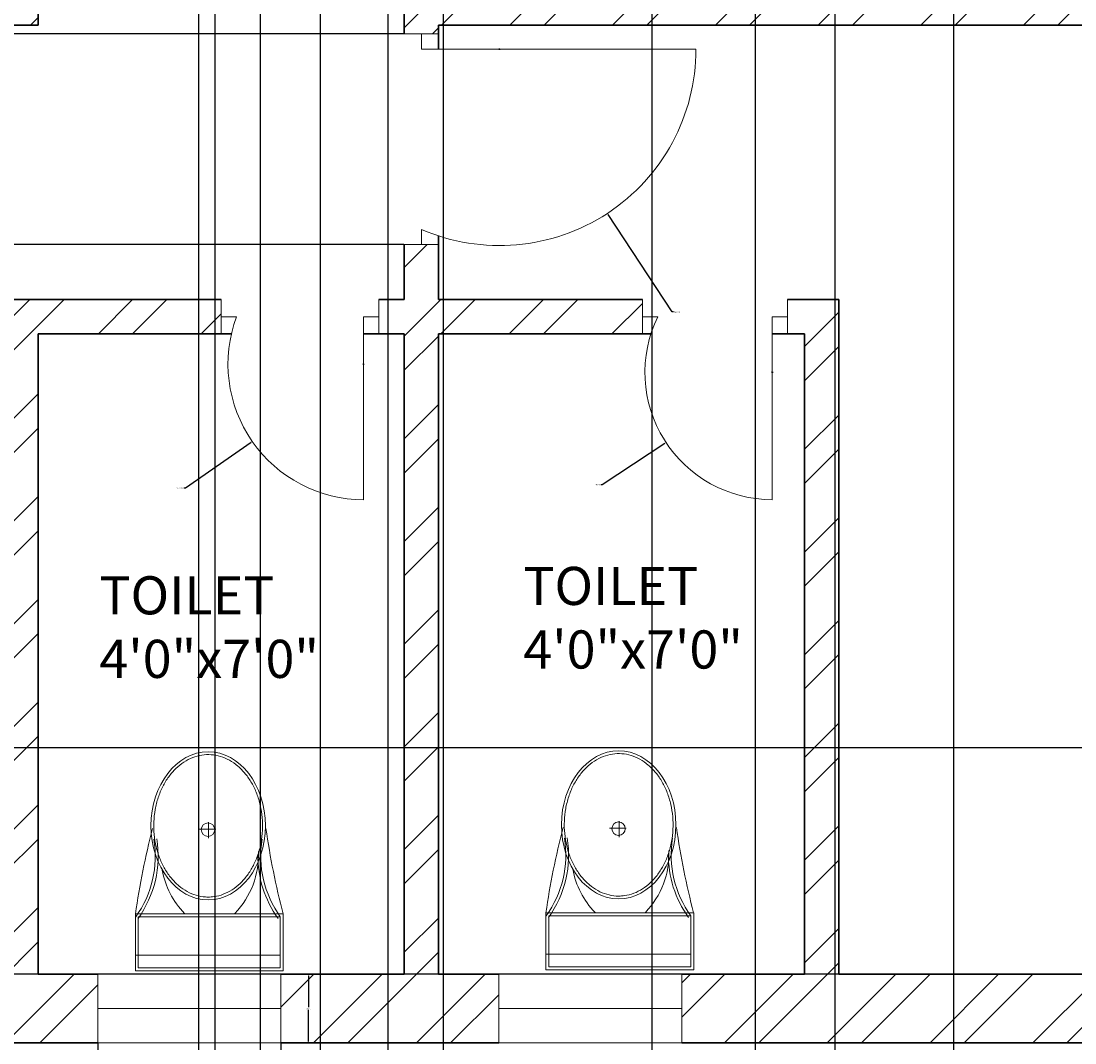
# Model space of a CAD drawing. Units: inches. Extents: x 1748 to 2382, y 1346 to 2284.
# Tile 4 of 26: x 2009 to 2147, y 1468 to 1602. Entities that reach past the tile are written whole.
import ezdxf

# ---------------------------------------------------------------- set-up
doc = ezdxf.new("R2010")
doc.units = ezdxf.units.IN
for name, color, linetype, lineweight in [('A-ANNO-DIMS', 2, 'Continuous', 18), ('A-AREA-IDEN', 7, 'Continuous', 18), ('A-DOOR', 21, 'Continuous', 18), ('A-FLOR-FIXT', 7, 'Continuous', 18), ('A-GLAZ', 191, 'Continuous', 18), ('A-WALL', 7, 'Continuous', 35), ('A-WALL-PATT', 9, 'Continuous', 13)]:
    doc.layers.add(name, color=color, linetype=linetype, lineweight=lineweight)
doc.styles.get("Standard").update_dxf_attribs({"font": 'arial.ttf'})
doc.dimstyles.get("Standard").update_dxf_attribs({"dimtxt": 0.18, "dimasz": 0.18, "dimexe": 0.18, "dimexo": 0.0625, "dimgap": 0.09, "dimtad": 0, "dimtih": 1, "dimtoh": 1, "dimdec": 4, "dimzin": 0, "dimdsep": 46, "dimtxsty": 'Standard', "dimcen": 0.09, "dimadec": 0, "dimazin": 0, "dimtfac": 1, "dimtdec": 4, "dimtofl": 0, "dimtmove": 0, "dimatfit": 3, "dimfxl": 1, "dimtolj": 1, "dimtzin": 0, "dimarcsym": 0})

# ---------------------------------------------------------------- blocks, each defined once
blk = doc.blocks.new('A$C31115884')
for p, q in [((257.5, 466.4), (257.5, 523.2)), ((283.1, 497.7), (223.4, 497.7)), ((0, 200), (0, 0)), ((520, 200), (0, 200)), ((10, 190), (10, 10)), ((510, 190), (10, 190)), ((510, 10), (510, 190)), ((520, 0), (520, 200)), ((510, 54.5), (0, 54.5)), ((10, 10), (510, 10)), ((0, 0), (520, 0))]:
    blk.add_line(p, q)
blk.add_circle((255.6, 496.4), 23.6)
for centre, radius, start, end in [((2777.7, -204.6), 2807, 165.4549, 171.7133), ((3237, 905), 2807, 188.2867, 194.5451), ((-294.5, 403.3), 364.7, 324.2091, 9.3499), ((-294.5, 403.3), 374.7, 324.2091, 9.3499), ((805.8, 403.3), 364.7, 170.6501, 215.7909), ((139.5, 406.2), 293.5, 315.8436, 2.6563), ((805.8, 403.3), 374.7, 179.2036, 215.7909), ((383.6, 406.2), 293.5, 190.2774, 224.1564)]:
    blk.add_arc(centre, radius, start, end)
blk.add_ellipse((256.2, 509.9), major_axis=(0, -260.7), ratio=0.772727)
blk.add_open_spline([(256.2, 259.2), (263.1, 259.2), (270, 259.7), (287.8, 262.3), (298.7, 265.1), (319.9, 273.1), (330.2, 278.4), (350.1, 291.1), (359.7, 298.7), (377.7, 315.9), (386.2, 325.5), (401.7, 346.6), (408.8, 358.1), (421.3, 382.5), (426.8, 395.5), (435.9, 422.4), (439.5, 436.4), (444.8, 465.1), (446.5, 479.7), (447.9, 509.2), (447.6, 524), (445, 553.3), (442.7, 567.8), (436.3, 596), (432.1, 609.7), (421.9, 636), (416, 648.6), (402.5, 672.1), (395, 683), (378.6, 703), (369.8, 712.1), (351.1, 728), (341.3, 734.8), (320.9, 746.2), (310.4, 750.7), (288.9, 757.3), (278, 759.4), (256, 761), (245, 760.6), (223.1, 757.2), (212.3, 754.3), (191.1, 746.1), (180.8, 740.7), (160.9, 727.8), (151.4, 720.1), (133.5, 702.7), (125.1, 693), (109.6, 671.7), (102.6, 660.2), (90.2, 635.7), (84.9, 622.7), (76, 595.6), (72.4, 581.6), (67.2, 552.9), (65.6, 538.2), (64.4, 508.8), (64.8, 494), (67.5, 464.7), (69.9, 450.2), (76.6, 422), (80.8, 408.3), (91.1, 382.2), (97.2, 369.7), (110.8, 346.3), (118.4, 335.4), (134.8, 315.6), (143.7, 306.7), (162.4, 290.9), (172.3, 284.2), (192.8, 273), (203.3, 268.6), (224.8, 262.2), (235.8, 260.2), (249.9, 259.3), (253, 259.2), (256.2, 259.2)], degree=3, knots=[0, 0, 0, 0, 0.110105, 0.110105, 0.285049, 0.285049, 0.459994, 0.459994, 0.634938, 0.634938, 0.809882, 0.809882, 0.984827, 0.984827, 1.159771, 1.159771, 1.334715, 1.334715, 1.50966, 1.50966, 1.684604, 1.684604, 1.859549, 1.859549, 2.034493, 2.034493, 2.209437, 2.209437, 2.384382, 2.384382, 2.559326, 2.559326, 2.73427, 2.73427, 2.909215, 2.909215, 3.084159, 3.084159, 3.259103, 3.259103, 3.434048, 3.434048, 3.608992, 3.608992, 3.783936, 3.783936, 3.958881, 3.958881, 4.133825, 4.133825, 4.30877, 4.30877, 4.483714, 4.483714, 4.658658, 4.658658, 4.833603, 4.833603, 5.008547, 5.008547, 5.183491, 5.183491, 5.358436, 5.358436, 5.53338, 5.53338, 5.708324, 5.708324, 5.883269, 5.883269, 6.058213, 6.058213, 6.233158, 6.233158, 6.283185, 6.283185, 6.283185, 6.283185])
blk = doc.blocks.new('WIN-24-DEEP')
for p, q in [((0, 9), (0, 0)), ((0, 9), (24, 9)), ((24, 4.5), (24, 9)), ((24, 9), (24, 0)), ((0, 0), (0, 4.5)), ((0, 4.5), (24, 4.5)), ((24, 0), (0, 0))]:
    blk.add_line(p, q)
blk = doc.blocks.new('*D32')
at = {"layer": 'A-ANNO-DIMS', "color": 0, "lineweight": -2, "transparency": 16777216}
for p, q in [((2018.79, 1467.79), (2018.79, 1464.07)), ((2042.79, 1467.79), (2042.79, 1464.07)), ((2018.97, 1464.25), (2029.67, 1464.25)), ((2042.61, 1464.25), (2031.91, 1464.25))]:
    blk.add_line(p, q, dxfattribs=at)
at = {"layer": 'A-ANNO-DIMS', "color": 0, "transparency": 16777216}
for points in [[(2018.97, 1464.28), (2018.97, 1464.22), (2018.79, 1464.25)], [(2042.61, 1464.28), (2042.61, 1464.22), (2042.79, 1464.25)]]:
    blk.add_solid(points, dxfattribs=at)
at = {"layer": 'Defpoints', "color": 0, "transparency": 16777216}
for p in [(2018.79, 1467.85), (2042.79, 1467.85), (2042.79, 1464.25)]:
    blk.add_point(p, dxfattribs=at)
at = {"layer": 'A-ANNO-DIMS', "color": 0, "transparency": 16777216, "insert": (2030.79, 1464.25), "char_height": 0.18, "attachment_point": 5}
blk.add_mtext('\\A1;WINDOW 24 TYP.', dxfattribs=at)
blk = doc.blocks.new('*D33')
at = {"layer": 'A-ANNO-DIMS', "color": 0, "lineweight": -2, "transparency": 16777216}
for p, q in [((2042.85, 1476.85), (2046.57, 1476.85)), ((2046.39, 1476.67), (2046.39, 1472.53)), ((2046.39, 1468.03), (2046.39, 1472.17)), ((2042.85, 1467.85), (2046.57, 1467.85))]:
    blk.add_line(p, q, dxfattribs=at)
at = {"layer": 'A-ANNO-DIMS', "color": 0, "transparency": 16777216}
for points in [[(2046.36, 1476.67), (2046.42, 1476.67), (2046.39, 1476.85)], [(2046.36, 1468.03), (2046.42, 1468.03), (2046.39, 1467.85)]]:
    blk.add_solid(points, dxfattribs=at)
at = {"layer": 'Defpoints', "color": 0, "transparency": 16777216}
for p in [(2042.79, 1476.85), (2046.39, 1476.85), (2042.79, 1467.85)]:
    blk.add_point(p, dxfattribs=at)
at = {"layer": 'A-ANNO-DIMS', "color": 0, "transparency": 16777216, "insert": (2046.39, 1472.35), "char_height": 0.18, "attachment_point": 5}
blk.add_mtext('\\A1;9 TYP.', dxfattribs=at)
blk = doc.blocks.new('*D36')
at = {"layer": 'A-ANNO-DIMS', "color": 0, "lineweight": -2, "transparency": 16777216}
for p, q in [((2031.96, 1970.29), (2031.96, 1360.47)), ((2130.96, 1970.29), (2130.96, 1360.47)), ((2032.14, 1360.65), (2081.24, 1360.65)), ((2130.78, 1360.65), (2081.68, 1360.65))]:
    blk.add_line(p, q, dxfattribs=at)
at = {"layer": 'A-ANNO-DIMS', "color": 0, "transparency": 16777216}
for points in [[(2032.14, 1360.68), (2032.14, 1360.62), (2031.96, 1360.65)], [(2130.78, 1360.68), (2130.78, 1360.62), (2130.96, 1360.65)]]:
    blk.add_solid(points, dxfattribs=at)
at = {"layer": 'Defpoints', "color": 0, "transparency": 16777216}
for p in [(2031.96, 1970.35), (2130.96, 1970.35), (2130.96, 1360.65)]:
    blk.add_point(p, dxfattribs=at)
at = {"layer": 'A-ANNO-DIMS', "color": 0, "transparency": 16777216, "insert": (2081.46, 1360.65), "char_height": 0.18, "attachment_point": 5}
blk.add_mtext('\\A1;99', dxfattribs=at)
blk = doc.blocks.new('*D51')
at = {"layer": 'A-ANNO-DIMS', "color": 0, "lineweight": -2, "transparency": 16777216}
for p, q in [((1968.44, 2223.79), (1968.44, 1360.47)), ((2040.07, 2223.79), (2040.07, 1360.47)), ((1968.62, 1360.65), (2003.86, 1360.65)), ((2039.89, 1360.65), (2004.65, 1360.65))]:
    blk.add_line(p, q, dxfattribs=at)
at = {"layer": 'A-ANNO-DIMS', "color": 0, "transparency": 16777216}
for points in [[(1968.62, 1360.68), (1968.62, 1360.62), (1968.44, 1360.65)], [(2039.89, 1360.68), (2039.89, 1360.62), (2040.07, 1360.65)]]:
    blk.add_solid(points, dxfattribs=at)
at = {"layer": 'Defpoints', "color": 0, "transparency": 16777216}
for p in [(1968.44, 2223.85), (2040.07, 2223.85), (2040.07, 1360.65)]:
    blk.add_point(p, dxfattribs=at)
at = {"layer": 'A-ANNO-DIMS', "color": 0, "transparency": 16777216, "insert": (2004.26, 1360.65), "char_height": 0.18, "attachment_point": 5}
blk.add_mtext('\\A1;71.62', dxfattribs=at)
blk = doc.blocks.new('*D52')
at = {"layer": 'A-ANNO-DIMS', "color": 0, "lineweight": -2, "transparency": 16777216}
for p, q in [((2064.07, 2223.79), (2064.07, 1360.47)), ((2091.4, 2223.79), (2091.4, 1360.47)), ((2064.25, 1360.65), (2077.34, 1360.65)), ((2091.22, 1360.65), (2078.13, 1360.65))]:
    blk.add_line(p, q, dxfattribs=at)
at = {"layer": 'A-ANNO-DIMS', "color": 0, "transparency": 16777216}
for points in [[(2064.25, 1360.68), (2064.25, 1360.62), (2064.07, 1360.65)], [(2091.22, 1360.68), (2091.22, 1360.62), (2091.4, 1360.65)]]:
    blk.add_solid(points, dxfattribs=at)
at = {"layer": 'Defpoints', "color": 0, "transparency": 16777216}
for p in [(2064.07, 2223.85), (2091.4, 2223.85), (2091.4, 1360.65)]:
    blk.add_point(p, dxfattribs=at)
at = {"layer": 'A-ANNO-DIMS', "color": 0, "transparency": 16777216, "insert": (2077.73, 1360.65), "char_height": 0.18, "attachment_point": 5}
blk.add_mtext('\\A1;27.33', dxfattribs=at)
blk = doc.blocks.new('*D53')
at = {"layer": 'A-ANNO-DIMS', "color": 0, "lineweight": -2, "transparency": 16777216}
for p, q in [((2115.4, 2223.79), (2115.4, 1360.47)), ((2167.02, 2223.79), (2167.02, 1360.47)), ((2115.58, 1360.65), (2140.81, 1360.65)), ((2166.84, 1360.65), (2141.6, 1360.65))]:
    blk.add_line(p, q, dxfattribs=at)
at = {"layer": 'A-ANNO-DIMS', "color": 0, "transparency": 16777216}
for points in [[(2115.58, 1360.68), (2115.58, 1360.62), (2115.4, 1360.65)], [(2166.84, 1360.68), (2166.84, 1360.62), (2167.02, 1360.65)]]:
    blk.add_solid(points, dxfattribs=at)
at = {"layer": 'Defpoints', "color": 0, "transparency": 16777216}
for p in [(2115.4, 2223.85), (2167.02, 2223.85), (2167.02, 1360.65)]:
    blk.add_point(p, dxfattribs=at)
at = {"layer": 'A-ANNO-DIMS', "color": 0, "transparency": 16777216, "insert": (2141.21, 1360.65), "char_height": 0.18, "attachment_point": 5}
blk.add_mtext('\\A1;51.62', dxfattribs=at)
blk = doc.blocks.new('*D54')
at = {"layer": 'A-ANNO-DIMS', "color": 0, "lineweight": -2, "transparency": 16777216}
for p, q in [((2288.4, 1506.57), (1779.88, 1506.57)), ((1780.06, 1506.39), (1780.06, 1491.89)), ((1780.06, 1477.03), (1780.06, 1491.53)), ((2288.4, 1476.85), (1779.88, 1476.85))]:
    blk.add_line(p, q, dxfattribs=at)
at = {"layer": 'A-ANNO-DIMS', "color": 0, "transparency": 16777216}
for points in [[(1780.03, 1506.39), (1780.09, 1506.39), (1780.06, 1506.57)], [(1780.03, 1477.03), (1780.09, 1477.03), (1780.06, 1476.85)]]:
    blk.add_solid(points, dxfattribs=at)
at = {"layer": 'Defpoints', "color": 0, "transparency": 16777216}
for p in [(1780.06, 1506.57), (2288.46, 1506.57), (2288.46, 1476.85)]:
    blk.add_point(p, dxfattribs=at)
at = {"layer": 'A-ANNO-DIMS', "color": 0, "transparency": 16777216, "insert": (1780.06, 1491.71), "char_height": 0.18, "attachment_point": 5}
blk.add_mtext('\\A1;29.716', dxfattribs=at)
blk = doc.blocks.new('*D61')
at = {"layer": 'A-ANNO-DIMS', "color": 0, "lineweight": -2, "transparency": 16777216}
for p, q in [((2047.92, 1854.79), (2047.92, 1360.47)), ((2104.96, 1854.79), (2104.96, 1360.47)), ((2048.1, 1360.65), (2076.04, 1360.65)), ((2104.78, 1360.65), (2076.83, 1360.65))]:
    blk.add_line(p, q, dxfattribs=at)
at = {"layer": 'A-ANNO-DIMS', "color": 0, "transparency": 16777216}
for points in [[(2048.1, 1360.68), (2048.1, 1360.62), (2047.92, 1360.65)], [(2104.78, 1360.68), (2104.78, 1360.62), (2104.96, 1360.65)]]:
    blk.add_solid(points, dxfattribs=at)
at = {"layer": 'Defpoints', "color": 0, "transparency": 16777216}
for p in [(2047.92, 1854.85), (2104.96, 1854.85), (2104.96, 1360.65)]:
    blk.add_point(p, dxfattribs=at)
at = {"layer": 'A-ANNO-DIMS', "color": 0, "transparency": 16777216, "insert": (2076.44, 1360.65), "char_height": 0.18, "attachment_point": 5}
blk.add_mtext('\\A1;57.04', dxfattribs=at)
blk = doc.blocks.new('*D78')
at = {"layer": 'A-ANNO-DIMS', "color": 0, "lineweight": -2, "transparency": 16777216}
for p, q in [((2034.13, 2132.54), (2034.13, 1360.47)), ((2056.8, 2127.06), (2056.8, 1360.47)), ((2034.31, 1360.65), (2045, 1360.65)), ((2056.62, 1360.65), (2045.93, 1360.65))]:
    blk.add_line(p, q, dxfattribs=at)
at = {"layer": 'A-ANNO-DIMS', "color": 0, "transparency": 16777216}
for points in [[(2034.31, 1360.68), (2034.31, 1360.62), (2034.13, 1360.65)], [(2056.62, 1360.68), (2056.62, 1360.62), (2056.8, 1360.65)]]:
    blk.add_solid(points, dxfattribs=at)
at = {"layer": 'Defpoints', "color": 0, "transparency": 16777216}
for p in [(2034.13, 2132.6), (2056.8, 2127.13), (2056.8, 1360.65)]:
    blk.add_point(p, dxfattribs=at)
at = {"layer": 'A-ANNO-DIMS', "color": 0, "transparency": 16777216, "insert": (2045.47, 1360.65), "char_height": 0.18, "attachment_point": 5}
blk.add_mtext('\\A1;22.663', dxfattribs=at)
blk = doc.blocks.new('*D80')
at = {"layer": 'A-ANNO-DIMS', "color": 0, "lineweight": -2, "transparency": 16777216}
for p, q in [((2058.9, 1600.19), (1779.88, 1600.19)), ((1780.06, 1600.01), (1780.06, 1586.55)), ((1780.06, 1572.73), (1780.06, 1586.19)), ((2058.9, 1572.55), (1779.88, 1572.55))]:
    blk.add_line(p, q, dxfattribs=at)
at = {"layer": 'A-ANNO-DIMS', "color": 0, "transparency": 16777216}
for points in [[(1780.03, 1600.01), (1780.09, 1600.01), (1780.06, 1600.19)], [(1780.03, 1572.73), (1780.09, 1572.73), (1780.06, 1572.55)]]:
    blk.add_solid(points, dxfattribs=at)
at = {"layer": 'Defpoints', "color": 0, "transparency": 16777216}
for p in [(1780.06, 1600.19), (2058.96, 1600.19), (2058.96, 1572.55)]:
    blk.add_point(p, dxfattribs=at)
at = {"layer": 'A-ANNO-DIMS', "color": 0, "transparency": 16777216, "insert": (1780.06, 1586.37), "char_height": 0.18, "attachment_point": 5}
blk.add_mtext('\\A1;27.637', dxfattribs=at)
blk = doc.blocks.new('*D86')
at = {"layer": 'A-ANNO-DIMS', "color": 0, "lineweight": -2, "transparency": 16777216}
for p, q in [((2071.36, 1598.19), (2071.54, 1598.19)), ((2071.45, 1598.1), (2071.45, 1598.28)), ((2094.07, 1563.73), (2085.69, 1576.5)), ((2094.25, 1563.73), (2094.07, 1563.73))]:
    blk.add_line(p, q, dxfattribs=at)
at = {"layer": 'A-ANNO-DIMS', "color": 0, "transparency": 16777216}
blk.add_solid([(2085.71, 1576.52), (2085.66, 1576.49), (2085.59, 1576.65)], dxfattribs=at)
at = {"layer": 'Defpoints', "color": 0, "transparency": 16777216}
for p in [(2071.45, 1598.19), (2085.59, 1576.65)]:
    blk.add_point(p, dxfattribs=at)
at = {"layer": 'A-ANNO-DIMS', "color": 0, "transparency": 16777216, "insert": (2094.73, 1563.73), "char_height": 0.18, "attachment_point": 5}
blk.add_mtext('\\A1;R25.76', dxfattribs=at)
blk = doc.blocks.new('*D92')
at = {"layer": 'A-ANNO-DIMS', "color": 0, "lineweight": -2, "transparency": 16777216}
for p, q in [((2053.54, 1556.89), (2053.72, 1556.89)), ((2053.63, 1556.8), (2053.63, 1556.98)), ((2030.25, 1540.65), (2038.87, 1546.64)), ((2030.07, 1540.65), (2030.25, 1540.65))]:
    blk.add_line(p, q, dxfattribs=at)
at = {"layer": 'A-ANNO-DIMS', "color": 0, "transparency": 16777216}
blk.add_solid([(2038.85, 1546.66), (2038.89, 1546.61), (2039.02, 1546.74)], dxfattribs=at)
at = {"layer": 'Defpoints', "color": 0, "transparency": 16777216}
for p in [(2053.63, 1556.89), (2039.02, 1546.74)]:
    blk.add_point(p, dxfattribs=at)
at = {"layer": 'A-ANNO-DIMS', "color": 0, "transparency": 16777216, "insert": (2029.52, 1540.65), "char_height": 0.18, "attachment_point": 5}
blk.add_mtext('\\A1;R17.788', dxfattribs=at)
blk = doc.blocks.new('*D96')
at = {"layer": 'A-ANNO-DIMS', "color": 0, "lineweight": -2, "transparency": 16777216}
for p, q in [((2107.13, 1555.81), (2107.31, 1555.81)), ((2107.22, 1555.72), (2107.22, 1555.9)), ((2084.92, 1541.07), (2093.13, 1546.5)), ((2084.74, 1541.07), (2084.92, 1541.07))]:
    blk.add_line(p, q, dxfattribs=at)
at = {"layer": 'A-ANNO-DIMS', "color": 0, "transparency": 16777216}
blk.add_solid([(2093.11, 1546.52), (2093.15, 1546.47), (2093.28, 1546.59)], dxfattribs=at)
at = {"layer": 'Defpoints', "color": 0, "transparency": 16777216}
for p in [(2107.22, 1555.81), (2093.28, 1546.59)]:
    blk.add_point(p, dxfattribs=at)
at = {"layer": 'A-ANNO-DIMS', "color": 0, "transparency": 16777216, "insert": (2084.28, 1541.07), "char_height": 0.18, "attachment_point": 5}
blk.add_mtext('\\A1;R16.71', dxfattribs=at)

msp = doc.modelspace()

# ---------------------------------------------------------------- hatches: boundary and pattern name
at = {"layer": 'A-WALL-PATT'}
h = msp.add_hatch(dxfattribs=at)
h.set_pattern_fill('ANSI32', color=256)
h.paths.add_polyline_path([(1908.4445, 2232.8497), (1821.9607, 2232.8497), (1821.9607, 2223.8497), (1865.4607, 2223.8497), (1865.4607, 2209.9185), (1869.9607, 2209.9185), (1869.9607, 2223.8497), (1908.4445, 2223.8497), (1908.4445, 2228.3497)])
h.paths.add_polyline_path([(2040.0683, 2232.8497), (1968.4445, 2232.8497), (1968.4445, 2223.8497), (2025.9607, 2223.8497), (2025.9607, 2130.3497), (2032.1341, 2130.3497), (2032.1341, 2132.5997), (2032.1341, 2134.8497), (2030.4607, 2134.8497), (2030.4607, 2223.8497), (2040.0683, 2223.8497)])
h.paths.add_polyline_path([(2091.3969, 2232.8497), (2064.0683, 2232.8497), (2064.0683, 2223.8497), (2078.4607, 2223.8497), (2078.4607, 2134.8497), (2051.1563, 2134.8497), (2051.1563, 2130.3497), (2078.4607, 2130.3497), (2078.4607, 2128.6813), (2082.9607, 2128.6813), (2082.9607, 2130.3497), (2086.1879, 2130.3497), (2086.1879, 2132.5997), (2086.1879, 2134.8497), (2082.9607, 2134.8497), (2082.9607, 2223.8497), (2091.3969, 2223.8497), (2091.3969, 2228.3497)])
h.paths.add_polyline_path([(2167.0164, 2232.8497), (2115.3969, 2232.8497), (2115.3969, 2223.8497), (2130.9607, 2223.8497), (2130.9607, 2134.8497), (2106.9607, 2134.8497), (2106.9607, 2130.3497), (2135.4607, 2130.3497), (2135.4607, 2223.8497), (2167.0164, 2223.8497), (2167.0164, 2228.3497)])
h.paths.add_polyline_path([(1869.9607, 2149.9185), (1865.4607, 2149.9185), (1865.4607, 2127.8942), (1869.9607, 2127.8942)])
h.paths.add_polyline_path([(2082.9607, 2104.4871), (2080.7107, 2104.4871), (2078.4607, 2104.4871), (2078.4607, 2103.8497), (1869.9607, 2103.8497), (1869.9607, 2108.6062), (1867.7107, 2108.6062), (1865.4607, 2108.6062), (1865.4607, 2103.8497), (1821.9607, 2103.8497), (1821.9607, 2099.3497), (1865.4607, 2099.3497), (1865.4607, 2094.7509), (1869.9607, 2094.7509), (1869.9607, 2099.3497), (2025.9607, 2099.3497), (2025.9607, 2096.4326), (2030.4607, 2096.4326), (2030.4607, 2099.3497), (2082.9607, 2099.3497)])
h.paths.add_polyline_path([(1928.9457, 1401.1212), (2176.8693, 1401.1212), (2176.8693, 1438.214), (1928.9457, 1438.214)], flags=9)
h.paths.add_polyline_path([(2122.2668, 2048.1927), (2177.9387, 2048.1927), (2177.9387, 2066.85), (2122.2668, 2066.85)], flags=9)
h.paths.add_polyline_path([(2272.688, 2153.8197), (2272.688, 2216.746), (2262.3845, 2216.746), (2262.3845, 2153.8197)], flags=9)
h.paths.add_polyline_path([(2157.2928, 2166.5593), (2196.3822, 2166.5593), (2196.3822, 2185.2167), (2157.2928, 2185.2167)], flags=9)
h.paths.add_polyline_path([(2089.3407, 2162.0698), (2124.3987, 2162.0698), (2124.3987, 2180.7272), (2089.3407, 2180.7272)], flags=9)
h.paths.add_polyline_path([(2037.4521, 2160.0913), (2072.5101, 2160.0913), (2072.5101, 2178.7486), (2037.4521, 2178.7486)], flags=9)
h.paths.add_polyline_path([(1884.7894, 2104.1554), (1923.6297, 2104.1554), (1923.6297, 2122.8127), (1884.7894, 2122.8127)], flags=9)
h.paths.add_polyline_path([(1851.2832, 2142.9749), (1851.2832, 2199.3051), (1840.9796, 2199.3051), (1840.9796, 2142.9749)], flags=9)
h.paths.add_polyline_path([(1844.8763, 2017.2834), (1844.8763, 2073.6136), (1834.5728, 2073.6136), (1834.5728, 2017.2834)], flags=9)
h.paths.add_polyline_path([(1897.1577, 2073.1279), (1935.9981, 2073.1279), (1935.9981, 2091.7853), (1897.1577, 2091.7853)], flags=9)
h.paths.add_polyline_path([(1952.3395, 1802.4231), (2008.0114, 1802.4231), (2008.0114, 1821.0805), (1952.3395, 1821.0805)], flags=9)
h.paths.add_polyline_path([(1978.8184, 1857.6841), (2017.7338, 1857.6841), (2017.7338, 1876.3415), (1978.8184, 1876.3415)], flags=9)
h.paths.add_polyline_path([(1979.6513, 1925.9516), (2008.8089, 1925.9516), (2008.8089, 1944.6089), (1979.6513, 1944.6089)], flags=9)
h.paths.add_polyline_path([(1838.5553, 1860.3527), (1877.3957, 1860.3527), (1877.3957, 1879.01), (1838.5553, 1879.01)], flags=9)
h.paths.add_polyline_path([(1883.9018, 1787.3013), (1883.9018, 1843.6315), (1873.5983, 1843.6315), (1873.5983, 1787.3013)], flags=9)
h.paths.add_polyline_path([(1873.7079, 1509.1938), (1873.7079, 1583.7709), (1863.4044, 1583.7709), (1863.4044, 1509.1938)], flags=9)
h.paths.add_polyline_path([(1916.2259, 1603.3681), (1955.0663, 1603.3681), (1955.0663, 1622.0254), (1916.2259, 1622.0254)], flags=9)
h.paths.add_polyline_path([(1876.3013, 1636.757), (1876.3013, 1693.0871), (1865.9978, 1693.0871), (1865.9978, 1636.757)], flags=9)
h.paths.add_polyline_path([(1921.3138, 1521.8316), (1964.0662, 1521.8316), (1964.0662, 1540.489), (1921.3138, 1540.489)], flags=9)
h.paths.add_polyline_path([(2017.5657, 1497.5078), (2046.7983, 1497.5078), (2046.7983, 1516.1651), (2017.5657, 1516.1651)], flags=9)
h.paths.add_polyline_path([(2066.8661, 1499.3902), (2096.0988, 1499.3902), (2096.0988, 1518.0475), (2066.8661, 1518.0475)], flags=9)
h.paths.add_polyline_path([(2155.4835, 1571.6596), (2198.2358, 1571.6596), (2198.2358, 1590.3169), (2155.4835, 1590.3169)], flags=9)
h.paths.add_polyline_path([(2094.9136, 1664.6812), (2150.5855, 1664.6812), (2150.5855, 1683.3386), (2094.9136, 1683.3386)], flags=9)
h.paths.add_polyline_path([(2257.6902, 1863.1628), (2269.8935, 1863.1628), (2269.8935, 1873.4664), (2257.6902, 1873.4664)], flags=9)
h.paths.add_polyline_path([(2164.0748, 1880.3089), (2189.8694, 1880.3089), (2189.8694, 1890.6124), (2164.0748, 1890.6124)], flags=9)
h.paths.add_polyline_path([(2239.4394, 1931.0585), (2268.8187, 1931.0585), (2268.8187, 1949.7159), (2239.4394, 1949.7159)], flags=9)
h = msp.add_hatch(dxfattribs=at)
h.set_pattern_fill('ANSI32', color=256)
h.paths.add_polyline_path([(2297.4607, 2232.8497), (2203.0164, 2232.8497), (2203.0164, 2223.8497), (2244.9607, 2223.8497), (2244.9607, 2127.8554), (2249.4607, 2127.8554), (2249.4607, 2223.8497), (2297.4607, 2223.8497)])
h.paths.add_polyline_path([(2297.4607, 2103.8497), (2249.4607, 2103.8497), (2249.4607, 2106.7497), (2247.2107, 2106.7497), (2244.9607, 2106.7497), (2244.9607, 2103.8497), (2130.9607, 2103.8497), (2130.9607, 2099.3497), (2288.4607, 2099.3497), (2288.4607, 2077.2008), (2297.4607, 2077.2008)])
h.paths.add_polyline_path([(1928.9457, 1401.1212), (2176.8693, 1401.1212), (2176.8693, 1438.214), (1928.9457, 1438.214)], flags=9)
h.paths.add_polyline_path([(2122.2668, 2048.1927), (2177.9387, 2048.1927), (2177.9387, 2066.85), (2122.2668, 2066.85)], flags=9)
h.paths.add_polyline_path([(2272.688, 2153.8197), (2272.688, 2216.746), (2262.3845, 2216.746), (2262.3845, 2153.8197)], flags=25)
h.paths.add_polyline_path([(2157.2928, 2166.5593), (2196.3822, 2166.5593), (2196.3822, 2185.2167), (2157.2928, 2185.2167)], flags=9)
h.paths.add_polyline_path([(2089.3407, 2162.0698), (2124.3987, 2162.0698), (2124.3987, 2180.7272), (2089.3407, 2180.7272)], flags=9)
h.paths.add_polyline_path([(2037.4521, 2160.0913), (2072.5101, 2160.0913), (2072.5101, 2178.7486), (2037.4521, 2178.7486)], flags=9)
h.paths.add_polyline_path([(1884.7894, 2104.1554), (1923.6297, 2104.1554), (1923.6297, 2122.8127), (1884.7894, 2122.8127)], flags=9)
h.paths.add_polyline_path([(1851.2832, 2142.9749), (1851.2832, 2199.3051), (1840.9796, 2199.3051), (1840.9796, 2142.9749)], flags=9)
h.paths.add_polyline_path([(1844.8763, 2017.2834), (1844.8763, 2073.6136), (1834.5728, 2073.6136), (1834.5728, 2017.2834)], flags=9)
h.paths.add_polyline_path([(1897.1577, 2073.1279), (1935.9981, 2073.1279), (1935.9981, 2091.7853), (1897.1577, 2091.7853)], flags=9)
h.paths.add_polyline_path([(1952.3395, 1802.4231), (2008.0114, 1802.4231), (2008.0114, 1821.0805), (1952.3395, 1821.0805)], flags=9)
h.paths.add_polyline_path([(1978.8184, 1857.6841), (2017.7338, 1857.6841), (2017.7338, 1876.3415), (1978.8184, 1876.3415)], flags=9)
h.paths.add_polyline_path([(1979.6513, 1925.9516), (2008.8089, 1925.9516), (2008.8089, 1944.6089), (1979.6513, 1944.6089)], flags=9)
h.paths.add_polyline_path([(1838.5553, 1860.3527), (1877.3957, 1860.3527), (1877.3957, 1879.01), (1838.5553, 1879.01)], flags=9)
h.paths.add_polyline_path([(1883.9018, 1787.3013), (1883.9018, 1843.6315), (1873.5983, 1843.6315), (1873.5983, 1787.3013)], flags=9)
h.paths.add_polyline_path([(1873.7079, 1509.1938), (1873.7079, 1583.7709), (1863.4044, 1583.7709), (1863.4044, 1509.1938)], flags=9)
h.paths.add_polyline_path([(1916.2259, 1603.3681), (1955.0663, 1603.3681), (1955.0663, 1622.0254), (1916.2259, 1622.0254)], flags=9)
h.paths.add_polyline_path([(1876.3013, 1636.757), (1876.3013, 1693.0871), (1865.9978, 1693.0871), (1865.9978, 1636.757)], flags=9)
h.paths.add_polyline_path([(1921.3138, 1521.8316), (1964.0662, 1521.8316), (1964.0662, 1540.489), (1921.3138, 1540.489)], flags=9)
h.paths.add_polyline_path([(2017.5657, 1497.5078), (2046.7983, 1497.5078), (2046.7983, 1516.1651), (2017.5657, 1516.1651)], flags=9)
h.paths.add_polyline_path([(2066.8661, 1499.3902), (2096.0988, 1499.3902), (2096.0988, 1518.0475), (2066.8661, 1518.0475)], flags=9)
h.paths.add_polyline_path([(2155.4835, 1571.6596), (2198.2358, 1571.6596), (2198.2358, 1590.3169), (2155.4835, 1590.3169)], flags=9)
h.paths.add_polyline_path([(2094.9136, 1664.6812), (2150.5855, 1664.6812), (2150.5855, 1683.3386), (2094.9136, 1683.3386)], flags=9)
h.paths.add_polyline_path([(2257.6902, 1863.1628), (2269.8935, 1863.1628), (2269.8935, 1873.4664), (2257.6902, 1873.4664)], flags=9)
h.paths.add_polyline_path([(2164.0748, 1880.3089), (2189.8694, 1880.3089), (2189.8694, 1890.6124), (2164.0748, 1890.6124)], flags=9)
h.paths.add_polyline_path([(2239.4394, 1931.0585), (2268.8187, 1931.0585), (2268.8187, 1949.7159), (2239.4394, 1949.7159)], flags=9)
h = msp.add_hatch(dxfattribs=at)
h.set_pattern_fill('ANSI32', color=256)
h.paths.add_polyline_path([(1919.6777, 1476.8497), (1900.6426, 1476.8497), (1900.6426, 1522.0826), (1898.3926, 1522.0826), (1896.1426, 1522.0826), (1896.1426, 1476.8497), (1857.1426, 1476.8497), (1857.1426, 1467.8497), (1896.1426, 1467.8497), (1919.6777, 1467.8497), (1919.6777, 1472.3497)])
h.paths.add_polyline_path([(2018.7873, 1472.3497), (2018.7873, 1476.8497), (2010.9607, 1476.8497), (2010.9607, 1560.8497), (2034.9607, 1560.8497), (2034.9607, 1565.3497), (2006.4607, 1565.3497), (2006.4607, 1476.8497), (1955.6777, 1476.8497), (1955.6777, 1467.8497), (2018.7873, 1467.8497)])
h.paths.add_polyline_path([(2152.3354, 1472.3497), (2152.3354, 1476.8497), (2115.9607, 1476.8497), (2115.9607, 1565.3497), (2109.2204, 1565.3497), (2109.2204, 1563.0997), (2109.2204, 1560.8497), (2111.4607, 1560.8497), (2111.4607, 1476.8497), (2095.3617, 1476.8497), (2095.3617, 1467.8497), (2152.3354, 1467.8497)])
h.paths.add_polyline_path([(2071.3617, 1476.8497), (2063.4607, 1476.8497), (2063.4607, 1560.8497), (2090.1865, 1560.8497), (2090.1865, 1565.3497), (2063.4607, 1565.3497), (2063.4607, 1572.5485), (2061.2107, 1572.5485), (2058.9607, 1572.5485), (2058.9607, 1565.3497), (2055.6281, 1565.3497), (2055.6281, 1560.8497), (2058.9607, 1560.8497), (2058.9607, 1476.8497), (2042.7873, 1476.8497), (2042.7873, 1467.8497), (2071.3617, 1467.8497), (2071.3617, 1472.3497)])
h.paths.add_polyline_path([(2297.4607, 1506.5652), (2288.4607, 1506.5652), (2288.4607, 1476.8497), (2212.3354, 1476.8497), (2212.3354, 1467.8497), (2297.4607, 1467.8497)])
h.paths.add_polyline_path([(2297.4607, 1645.3038), (2288.4607, 1645.3038), (2288.4607, 1605.8497), (2058.9607, 1605.8497), (2058.9607, 1600.1857), (2061.2107, 1600.1857), (2063.4607, 1600.1857), (2063.4607, 1601.3497), (2288.4607, 1601.3497), (2288.4607, 1566.5652), (2297.4607, 1566.5652)])
h.paths.add_polyline_path([(2010.9607, 1609.0561), (2008.7107, 1609.0561), (2006.4607, 1609.0561), (2006.4607, 1605.8497), (1900.6426, 1605.8497), (1900.6426, 1609.7171), (1898.3926, 1609.7171), (1896.1426, 1609.7171), (1896.1426, 1605.8497), (1857.1426, 1605.8497), (1857.1426, 1601.3497), (1896.1426, 1601.3497), (1896.1426, 1542.5447), (1900.6426, 1542.5447), (1900.6426, 1601.3497), (2010.9607, 1601.3497)])
h.paths.add_polyline_path([(1928.9457, 1401.1212), (2176.8693, 1401.1212), (2176.8693, 1438.214), (1928.9457, 1438.214)], flags=9)
h.paths.add_polyline_path([(2122.2668, 2048.1927), (2177.9387, 2048.1927), (2177.9387, 2066.85), (2122.2668, 2066.85)], flags=9)
h.paths.add_polyline_path([(2272.688, 2153.8197), (2272.688, 2216.746), (2262.3845, 2216.746), (2262.3845, 2153.8197)], flags=9)
h.paths.add_polyline_path([(2157.2928, 2166.5593), (2196.3822, 2166.5593), (2196.3822, 2185.2167), (2157.2928, 2185.2167)], flags=9)
h.paths.add_polyline_path([(2089.3407, 2162.0698), (2124.3987, 2162.0698), (2124.3987, 2180.7272), (2089.3407, 2180.7272)], flags=9)
h.paths.add_polyline_path([(2037.4521, 2160.0913), (2072.5101, 2160.0913), (2072.5101, 2178.7486), (2037.4521, 2178.7486)], flags=9)
h.paths.add_polyline_path([(1884.7894, 2104.1554), (1923.6297, 2104.1554), (1923.6297, 2122.8127), (1884.7894, 2122.8127)], flags=9)
h.paths.add_polyline_path([(1851.2832, 2142.9749), (1851.2832, 2199.3051), (1840.9796, 2199.3051), (1840.9796, 2142.9749)], flags=9)
h.paths.add_polyline_path([(1844.8763, 2017.2834), (1844.8763, 2073.6136), (1834.5728, 2073.6136), (1834.5728, 2017.2834)], flags=9)
h.paths.add_polyline_path([(1897.1577, 2073.1279), (1935.9981, 2073.1279), (1935.9981, 2091.7853), (1897.1577, 2091.7853)], flags=9)
h.paths.add_polyline_path([(1952.3395, 1802.4231), (2008.0114, 1802.4231), (2008.0114, 1821.0805), (1952.3395, 1821.0805)], flags=9)
h.paths.add_polyline_path([(1978.8184, 1857.6841), (2017.7338, 1857.6841), (2017.7338, 1876.3415), (1978.8184, 1876.3415)], flags=9)
h.paths.add_polyline_path([(1979.6513, 1925.9516), (2008.8089, 1925.9516), (2008.8089, 1944.6089), (1979.6513, 1944.6089)], flags=9)
h.paths.add_polyline_path([(1838.5553, 1860.3527), (1877.3957, 1860.3527), (1877.3957, 1879.01), (1838.5553, 1879.01)], flags=9)
h.paths.add_polyline_path([(1883.9018, 1787.3013), (1883.9018, 1843.6315), (1873.5983, 1843.6315), (1873.5983, 1787.3013)], flags=9)
h.paths.add_polyline_path([(1873.7079, 1509.1938), (1873.7079, 1583.7709), (1863.4044, 1583.7709), (1863.4044, 1509.1938)], flags=9)
h.paths.add_polyline_path([(1916.2259, 1603.3681), (1955.0663, 1603.3681), (1955.0663, 1622.0254), (1916.2259, 1622.0254)], flags=9)
h.paths.add_polyline_path([(1876.3013, 1636.757), (1876.3013, 1693.0871), (1865.9978, 1693.0871), (1865.9978, 1636.757)], flags=9)
h.paths.add_polyline_path([(1921.3138, 1521.8316), (1964.0662, 1521.8316), (1964.0662, 1540.489), (1921.3138, 1540.489)], flags=9)
h.paths.add_polyline_path([(2017.5657, 1497.5078), (2046.7983, 1497.5078), (2046.7983, 1516.1651), (2017.5657, 1516.1651)], flags=9)
h.paths.add_polyline_path([(2066.8661, 1499.3902), (2096.0988, 1499.3902), (2096.0988, 1518.0475), (2066.8661, 1518.0475)], flags=9)
h.paths.add_polyline_path([(2155.4835, 1571.6596), (2198.2358, 1571.6596), (2198.2358, 1590.3169), (2155.4835, 1590.3169)], flags=25)
h.paths.add_polyline_path([(2094.9136, 1664.6812), (2150.5855, 1664.6812), (2150.5855, 1683.3386), (2094.9136, 1683.3386)], flags=9)
h.paths.add_polyline_path([(2257.6902, 1863.1628), (2269.8935, 1863.1628), (2269.8935, 1873.4664), (2257.6902, 1873.4664)], flags=9)
h.paths.add_polyline_path([(2164.0748, 1880.3089), (2189.8694, 1880.3089), (2189.8694, 1890.6124), (2164.0748, 1890.6124)], flags=9)
h.paths.add_polyline_path([(2239.4394, 1931.0585), (2268.8187, 1931.0585), (2268.8187, 1949.7159), (2239.4394, 1949.7159)], flags=9)

# ---------------------------------------------------------------- linework, layer by layer
at = {"layer": 'A-DOOR'}
for p, q in [((2063.4607, 1600.1857), (2058.9607, 1600.1857)), ((2058.9607, 1600.1857), (2061.2107, 1600.1857)), ((2061.2107, 1600.1857), (2061.2107, 1598.1857)), ((2061.2107, 1598.1857), (2097.2107, 1598.1857)), ((2061.2107, 1572.5485), (2061.2107, 1574.5485)), ((2058.9607, 1572.5485), (2063.4607, 1572.5485)), ((2063.4607, 1572.5485), (2061.2107, 1572.5485)), ((2034.9607, 1560.8497), (2034.9607, 1565.3497)), ((2034.9607, 1565.3497), (2034.9607, 1563.0997)), ((2055.6281, 1565.3497), (2055.6281, 1560.8497)), ((2090.1865, 1560.8497), (2090.1865, 1565.3497)), ((2090.1865, 1565.3497), (2090.1865, 1563.0997)), ((2109.2204, 1560.8497), (2109.2204, 1565.3497)), ((2109.2204, 1565.3497), (2109.2204, 1563.0997)), ((2034.9607, 1563.0997), (2036.9607, 1563.0997)), ((2055.6281, 1563.0997), (2053.6281, 1563.0997)), ((2053.6281, 1563.0997), (2053.6281, 1539.0997)), ((2055.6281, 1560.8497), (2055.6281, 1563.0997)), ((2090.1865, 1563.0997), (2092.1865, 1563.0997)), ((2109.2204, 1563.0997), (2107.2204, 1563.0997)), ((2107.2204, 1563.0997), (2107.2204, 1539.0997))]:
    msp.add_line(p, q, dxfattribs=at)
for centre, radius, start, end in [((2071.4507, 1598.1857), 25.76, 246.5769, 0), ((2053.6281, 1556.8872), 17.7876, 159.558264, 270), ((2107.2204, 1555.8084), 16.7087, 154.127235, 270)]:
    msp.add_arc(centre, radius, start, end, dxfattribs=at)
at = {"layer": 'A-WALL'}
for p, q in [((2010.9607, 1609.0561), (2010.9607, 1601.3497)), ((2058.9607, 1605.8497), (2058.9607, 1600.1857)), ((1900.6426, 1601.3497), (2010.9607, 1601.3497)), ((2063.4607, 1601.3497), (2288.4607, 1601.3497)), ((2063.4607, 1601.3497), (2063.4607, 1598.1857)), ((2063.4607, 1573.6962), (2063.4607, 1565.3497)), ((2058.9607, 1572.5485), (2058.9607, 1565.3497)), ((2006.4607, 1565.3497), (2034.9607, 1565.3497)), ((2055.6281, 1565.3497), (2058.9607, 1565.3497)), ((2063.4607, 1565.3497), (2090.1865, 1565.3497)), ((2109.2204, 1565.3497), (2115.9607, 1565.3497)), ((2115.9607, 1565.3497), (2115.9607, 1476.8497)), ((2010.9607, 1560.8497), (2036.2875, 1560.8497)), ((2010.9607, 1560.8497), (2010.9607, 1476.8497)), ((2053.6281, 1560.8497), (2058.9607, 1560.8497)), ((2058.9607, 1560.8497), (2058.9607, 1476.8497)), ((2063.4607, 1560.8497), (2091.2903, 1560.8497)), ((2063.4607, 1560.8497), (2063.4607, 1476.8497)), ((2107.2204, 1560.8497), (2111.4607, 1560.8497)), ((2111.4607, 1560.8497), (2111.4607, 1476.8497)), ((2010.9607, 1476.8497), (2018.7873, 1476.8497)), ((2042.7873, 1476.8497), (2058.9607, 1476.8497)), ((2063.4607, 1476.8497), (2071.3617, 1476.8497)), ((2095.3617, 1476.8497), (2111.4607, 1476.8497)), ((2115.9607, 1476.8497), (2152.3354, 1476.8497)), ((1955.6777, 1467.8497), (2018.7873, 1467.8497)), ((2042.7873, 1467.8497), (2071.3617, 1467.8497)), ((2095.3617, 1467.8497), (2152.3354, 1467.8497))]:
    msp.add_line(p, q, dxfattribs=at)

# ---------------------------------------------------------------- block references
at = {"layer": 'A-FLOR-FIXT', "xscale": 0.0372717239612423, "yscale": 0.0372717239612423, "zscale": 0.0372717239612423}
for p in [(2023.6967, 1477.3212), (2077.5249, 1477.448)]:
    msp.add_blockref('A$C31115884', p, dxfattribs=at)
at = {"layer": 'A-GLAZ'}
msp.add_blockref('WIN-24-DEEP', (2018.787, 1467.85), dxfattribs=at)
at = {"layer": 'A-GLAZ', "rotation": 180}
msp.add_blockref('WIN-24-DEEP', (2095.362, 1476.8493), dxfattribs=at)

# ---------------------------------------------------------------- texts
at = {"layer": 'A-AREA-IDEN', "char_height": 5, "attachment_point": 1}
for width, insert in [(164.087299, (2074.5666, 1530.2885)), (103.104972, (2018.9794, 1529.0574))]:
    msp.add_mtext_dynamic_manual_height_columns('TOILET\\P4\'0"x7\'0"', width=width, gutter_width=12.5, heights=[0], dxfattribs=dict(at, insert=insert))

# ---------------------------------------------------------------- dimensions: what is measured, and where the dimension line sits
at = {"layer": 'A-ANNO-DIMS'}
for base, p1, p2, override, picture, middle in [((2040.0683, 1360.6451), (1968.4445, 2223.8497), (2040.0683, 2223.8497), {"dimdec": 2, "dimlfac": 1, "dimrnd": 0, "dimzin": 0, "dimdsep": 46, "dimlunit": 2}, '*D51', (2004.2564, 1360.6451)), ((2091.3969, 1360.6451), (2064.0683, 2223.8497), (2091.3969, 2223.8497), {"dimdec": 2, "dimlfac": 1, "dimrnd": 0, "dimzin": 0, "dimdsep": 46, "dimlunit": 2}, '*D52', (2077.7326, 1360.6451)), ((2167.0164, 1360.6451), (2115.3969, 2223.8497), (2167.0164, 2223.8497), {"dimdec": 2, "dimlfac": 1, "dimrnd": 0, "dimzin": 0, "dimdsep": 46, "dimlunit": 2}, '*D53', (2141.2066, 1360.6451)), ((2056.7974, 1360.6451), (2034.1341, 2132.5997), (2056.7974, 2127.1257), {"dimdec": 3, "dimlfac": 1, "dimrnd": 0, "dimzin": 0, "dimdsep": 46, "dimlunit": 2}, '*D78', (2045.4658, 1360.6451)), ((2130.9607, 1360.6451), (2031.9607, 1970.3497), (2130.9607, 1970.3497), {"dimdec": 0, "dimlfac": 1, "dimrnd": 0, "dimzin": 0, "dimdsep": 46, "dimlunit": 2}, '*D36', (2081.4607, 1360.6451)), ((2104.9565, 1360.6451), (2047.917, 1854.8497), (2104.9565, 1854.8497), {"dimdec": 2, "dimlfac": 1, "dimrnd": 0, "dimzin": 0, "dimdsep": 46, "dimlunit": 2}, '*D61', (2076.4368, 1360.6451))]:
    dim = msp.add_linear_dim(base=base, p1=p1, p2=p2, dimstyle='Standard', override=override, dxfattribs=at)
    dim.commit()
    dim.dimension.update_dxf_attribs({"geometry": picture, "text_midpoint": middle})
for base, p1, p2, picture, middle in [((1780.0607, 1600.1857), (2058.9607, 1572.5485), (2058.9607, 1600.1857), '*D80', (1780.0607, 1586.3671)), ((1780.06066, 1506.56516), (2288.46066, 1476.84965), (2288.46066, 1506.56516), '*D54', (1780.06066, 1491.7074))]:
    dim = msp.add_linear_dim(base=base, p1=p1, p2=p2, angle=90, dimstyle='Standard', override={"dimdec": 3, "dimlfac": 1, "dimrnd": 0, "dimzin": 0, "dimdsep": 46, "dimlunit": 2}, dxfattribs=at)
    dim.commit()
    dim.dimension.update_dxf_attribs({"geometry": picture, "text_midpoint": middle})
for center, mpoint, override, picture, middle in [((2071.4507, 1598.1857), (2085.5888, 1576.6522), {"dimdec": 2, "dimlfac": 1, "dimrnd": 0, "dimzin": 0, "dimdsep": 46, "dimlunit": 2}, '*D86', (2094.7315, 1563.7322)), ((2053.6281, 1556.8872), (2039.0181, 1546.7411), {"dimdec": 3, "dimlfac": 1, "dimrnd": 0, "dimzin": 0, "dimdsep": 46, "dimlunit": 2}, '*D92', (2029.5221, 1540.6533)), ((2107.2204, 1555.8084), (2093.2817, 1546.5947), {"dimdec": 2, "dimlfac": 1, "dimrnd": 0, "dimzin": 0, "dimdsep": 46, "dimlunit": 2}, '*D96', (2084.2759, 1541.0664))]:
    dim = msp.add_radius_dim(center=center, mpoint=mpoint, dimstyle='Standard', override=override, dxfattribs=at)
    dim.commit()
    dim.dimension.update_dxf_attribs({"geometry": picture, "text_midpoint": middle, "dimtype": 164})
dim = msp.add_linear_dim(base=(2046.3873, 1476.8497), p1=(2042.7873, 1467.8497), p2=(2042.7873, 1476.8497), angle=90, text='<> TYP.', dimstyle='Standard', override={"dimdec": 0, "dimlfac": 1, "dimrnd": 0, "dimzin": 0, "dimdsep": 46, "dimlunit": 2}, dxfattribs=at)
dim.commit()
dim.dimension.update_dxf_attribs({"geometry": '*D33', "text_midpoint": (2046.3873, 1472.3497)})
dim = msp.add_linear_dim(base=(2042.7873, 1464.2497), p1=(2018.7873, 1467.8497), p2=(2042.7873, 1467.8497), text='WINDOW <> TYP.', dimstyle='Standard', override={"dimdec": 0, "dimlfac": 1, "dimrnd": 0, "dimzin": 0, "dimdsep": 46, "dimlunit": 2}, dxfattribs=at)
dim.commit()
dim.dimension.update_dxf_attribs({"geometry": '*D32', "text_midpoint": (2030.7873, 1464.2497)})

doc.saveas('drawing.dxf')
